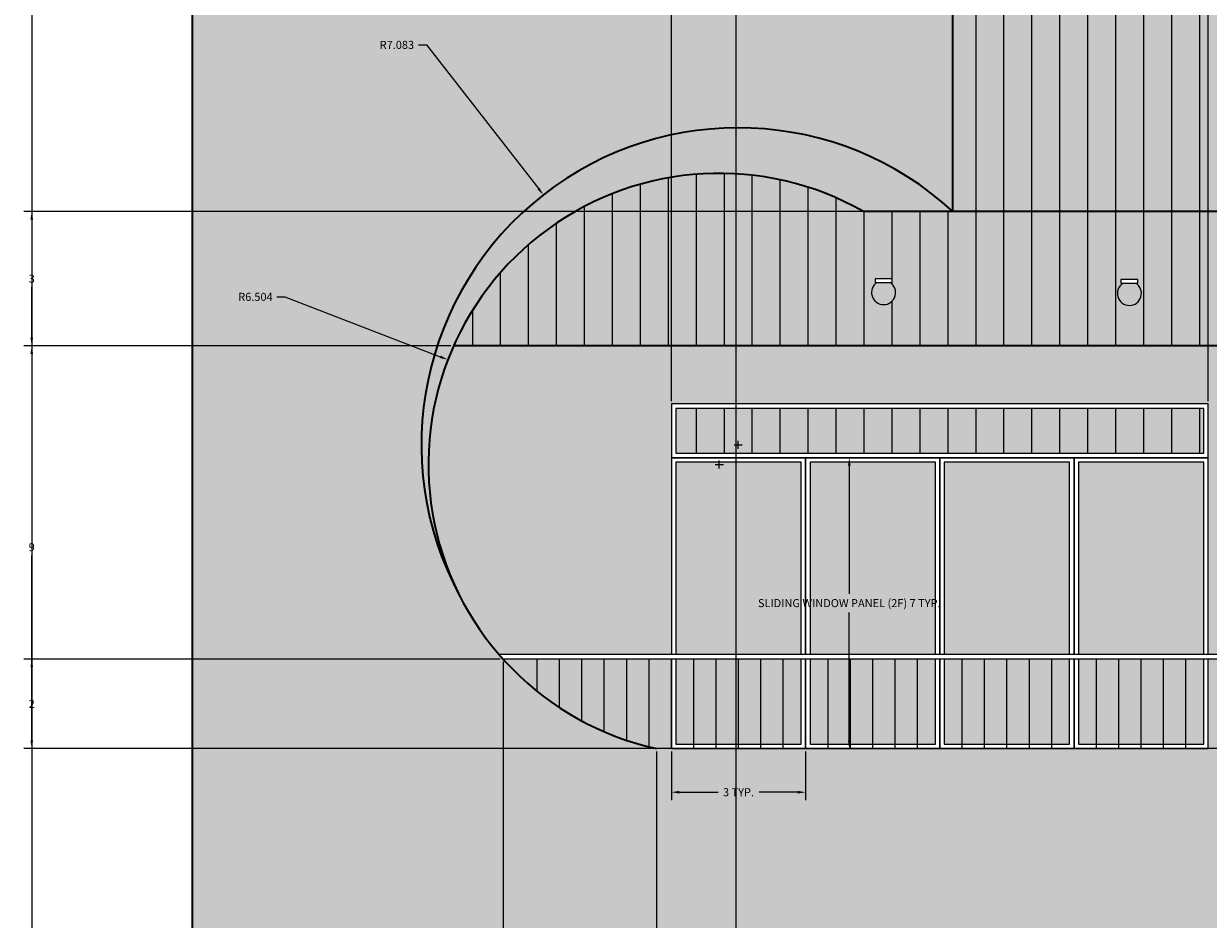
# Model space of a CAD drawing. Units: inches. Extents: x 18 to 59.8, y 2.7 to 81.2.
# Tile 7 of 9: x 18.1 to 44.6, y 45.6 to 65.6. Entities that reach past the tile are written whole.
import ezdxf

# ---------------------------------------------------------------- set-up
doc = ezdxf.new("R2010")
doc.units = ezdxf.units.IN
doc.header["$MEASUREMENT"] = 0
for name, color, linetype, lineweight in [('A-ANNO-DIMS', 2, 'Continuous', 18), ('A-ELEV', 7, 'Continuous', 35), ('A-ELEV-PATT', 8, 'Continuous', 13), ('A-ELEV-RAIL', 7, 'Continuous', 18), ('A-GLAZ', 4, 'Continuous', 25), ('E-LITE', 2, 'Continuous', 18)]:
    doc.layers.add(name, color=color, linetype=linetype, lineweight=lineweight)
doc.styles.get("Standard").update_dxf_attribs({"font": 'arial.ttf'})
doc.dimstyles.get("Standard").update_dxf_attribs({"dimtxt": 0.18, "dimasz": 0.18, "dimexe": 0.18, "dimexo": 0.0625, "dimgap": 0.09, "dimtad": 0, "dimtih": 1, "dimtoh": 1, "dimdec": 1, "dimzin": 0, "dimdsep": 46, "dimlunit": 3, "dimtxsty": 'Standard', "dimcen": 0.09, "dimadec": 0, "dimazin": 0, "dimtfac": 1, "dimtdec": 1, "dimtofl": 0, "dimtmove": 0, "dimatfit": 3, "dimfxl": 1, "dimtolj": 1, "dimtzin": 0, "dimarcsym": 0})

# ---------------------------------------------------------------- blocks, each defined once
blk = doc.blocks.new('LIGHT-CEILING-SPOT')
blk.add_lwpolyline([(0.079, 0.497), (0.459, 0.497), (0.459, 0.579), (0.079, 0.579)], close=True)
blk.add_arc((0.269, 0.269), 0.269, 122.0956, 57.9044)
blk = doc.blocks.new('WIN-SLIDING-PANEL-2F')
for points in [[(3, 2.1), (3, 6.5), (0, 6.5), (0, 2.1)], [(2.9, 2.1), (2.9, 6.4), (0.1, 6.4), (0.1, 2.1)], [(0, 2), (0, 0), (3, 0), (3, 2)], [(0.1, 2), (0.1, 0.1), (2.9, 0.1), (2.9, 2)]]:
    blk.add_lwpolyline(points)
blk = doc.blocks.new('*D6')
at = {"layer": 'A-ANNO-DIMS', "color": 0, "lineweight": -2, "transparency": 16777216}
for p, q in [((35.63, 55.941), (36.722, 55.941)), ((36.542, 55.761), (36.542, 52.899)), ((36.542, 49.621), (36.542, 52.483)), ((35.63, 49.441), (36.722, 49.441))]:
    blk.add_line(p, q, dxfattribs=at)
at = {"layer": 'A-ANNO-DIMS', "color": 0, "transparency": 16777216}
for points in [[(36.512, 55.761), (36.572, 55.761), (36.542, 55.941)], [(36.512, 49.621), (36.572, 49.621), (36.542, 49.441)]]:
    blk.add_solid(points, dxfattribs=at)
at = {"layer": 'Defpoints', "color": 0, "transparency": 16777216}
for p in [(35.567, 55.941), (36.542, 55.941), (35.567, 49.441)]:
    blk.add_point(p, dxfattribs=at)
at = {"layer": 'A-ANNO-DIMS', "color": 0, "transparency": 16777216, "insert": (36.542, 52.691), "char_height": 0.18, "attachment_point": 5}
blk.add_mtext('\\A1;SLIDING WINDOW PANEL (2F) 7 TYP.', dxfattribs=at)
blk = doc.blocks.new('*D7')
at = {"layer": 'A-ANNO-DIMS', "color": 0, "lineweight": -2, "transparency": 16777216}
for p, q in [((32.567, 49.378), (32.567, 48.286)), ((35.567, 49.378), (35.567, 48.286)), ((32.747, 48.466), (33.609, 48.466)), ((35.387, 48.466), (34.525, 48.466))]:
    blk.add_line(p, q, dxfattribs=at)
at = {"layer": 'A-ANNO-DIMS', "color": 0, "transparency": 16777216}
for points in [[(32.747, 48.496), (32.747, 48.436), (32.567, 48.466)], [(35.387, 48.496), (35.387, 48.436), (35.567, 48.466)]]:
    blk.add_solid(points, dxfattribs=at)
at = {"layer": 'Defpoints', "color": 0, "transparency": 16777216}
for p in [(32.567, 49.441), (35.567, 49.441), (35.567, 48.466)]:
    blk.add_point(p, dxfattribs=at)
at = {"layer": 'A-ANNO-DIMS', "color": 0, "transparency": 16777216, "insert": (34.067, 48.466), "char_height": 0.18, "attachment_point": 5}
blk.add_mtext('\\A1;3 TYP.', dxfattribs=at)
blk = doc.blocks.new('*D14')
at = {"layer": 'A-ANNO-DIMS', "color": 0, "lineweight": -2, "transparency": 16777216}
for p, q in [((21.797, 77.441), (18.09, 77.441)), ((18.27, 77.261), (18.27, 42.121)), ((18.27, 6.621), (18.27, 41.76)), ((21.797, 6.441), (18.09, 6.441))]:
    blk.add_line(p, q, dxfattribs=at)
at = {"layer": 'A-ANNO-DIMS', "color": 0, "transparency": 16777216}
for points in [[(18.24, 77.261), (18.3, 77.261), (18.27, 77.441)], [(18.24, 6.621), (18.3, 6.621), (18.27, 6.441)]]:
    blk.add_solid(points, dxfattribs=at)
at = {"layer": 'Defpoints', "color": 0, "transparency": 16777216}
for p in [(18.27, 77.441), (21.86, 77.441), (21.86, 6.441)]:
    blk.add_point(p, dxfattribs=at)
at = {"layer": 'A-ANNO-DIMS', "color": 0, "transparency": 16777216, "insert": (18.27, 41.941), "char_height": 0.18, "attachment_point": 5}
blk.add_mtext('\\A1;71', dxfattribs=at)
blk = doc.blocks.new('*D51')
at = {"layer": 'A-ANNO-DIMS', "color": 0, "lineweight": -2, "transparency": 16777216}
for p, q in [((34.012, 44.503), (34.012, 81.211)), ((34.192, 81.031), (40.98, 81.031)), ((48.68, 81.031), (41.891, 81.031)), ((48.86, 43.503), (48.86, 81.211))]:
    blk.add_line(p, q, dxfattribs=at)
at = {"layer": 'A-ANNO-DIMS', "color": 0, "transparency": 16777216}
for points in [[(34.192, 81.061), (34.192, 81.001), (34.012, 81.031)], [(48.68, 81.061), (48.68, 81.001), (48.86, 81.031)]]:
    blk.add_solid(points, dxfattribs=at)
at = {"layer": 'Defpoints', "color": 0, "transparency": 16777216}
for p in [(48.86, 81.031), (34.012, 44.441), (48.86, 43.441)]:
    blk.add_point(p, dxfattribs=at)
at = {"layer": 'A-ANNO-DIMS', "color": 0, "transparency": 16777216, "insert": (41.436, 81.031), "char_height": 0.18, "attachment_point": 5}
blk.add_mtext('\\A1;14.848', dxfattribs=at)
blk = doc.blocks.new('*D59')
at = {"layer": 'A-ANNO-DIMS', "color": 0, "lineweight": -2, "transparency": 16777216}
for p, q in [((27.636, 58.441), (18.09, 58.441)), ((18.27, 58.261), (18.27, 54.123)), ((18.27, 49.621), (18.27, 53.759)), ((32.171, 49.441), (18.09, 49.441))]:
    blk.add_line(p, q, dxfattribs=at)
at = {"layer": 'A-ANNO-DIMS', "color": 0, "transparency": 16777216}
for points in [[(18.24, 58.261), (18.3, 58.261), (18.27, 58.441)], [(18.24, 49.621), (18.3, 49.621), (18.27, 49.441)]]:
    blk.add_solid(points, dxfattribs=at)
at = {"layer": 'Defpoints', "color": 0, "transparency": 16777216}
for p in [(18.27, 58.441), (27.699, 58.441), (32.234, 49.441)]:
    blk.add_point(p, dxfattribs=at)
at = {"layer": 'A-ANNO-DIMS', "color": 0, "transparency": 16777216, "insert": (18.27, 53.941), "char_height": 0.18, "attachment_point": 5}
blk.add_mtext('\\A1;9', dxfattribs=at)
blk = doc.blocks.new('*D60')
at = {"layer": 'A-ANNO-DIMS', "color": 0, "lineweight": -2, "transparency": 16777216}
for p, q in [((38.797, 61.441), (18.09, 61.441)), ((18.27, 61.261), (18.27, 60.123)), ((18.27, 58.621), (18.27, 59.759)), ((27.636, 58.441), (18.09, 58.441))]:
    blk.add_line(p, q, dxfattribs=at)
at = {"layer": 'A-ANNO-DIMS', "color": 0, "transparency": 16777216}
for points in [[(18.24, 61.261), (18.3, 61.261), (18.27, 61.441)], [(18.24, 58.621), (18.3, 58.621), (18.27, 58.441)]]:
    blk.add_solid(points, dxfattribs=at)
at = {"layer": 'Defpoints', "color": 0, "transparency": 16777216}
for p in [(18.27, 61.441), (38.86, 61.441), (27.699, 58.441)]:
    blk.add_point(p, dxfattribs=at)
at = {"layer": 'A-ANNO-DIMS', "color": 0, "transparency": 16777216, "insert": (18.27, 59.941), "char_height": 0.18, "attachment_point": 5}
blk.add_mtext('\\A1;3', dxfattribs=at)
blk = doc.blocks.new('*D61')
at = {"layer": 'A-ANNO-DIMS', "color": 0, "lineweight": -2, "transparency": 16777216}
for p, q in [((32.234, 49.378), (32.234, 2.671)), ((47.86, 49.378), (47.86, 2.671)), ((32.414, 2.851), (39.592, 2.851)), ((47.68, 2.851), (40.502, 2.851))]:
    blk.add_line(p, q, dxfattribs=at)
at = {"layer": 'A-ANNO-DIMS', "color": 0, "transparency": 16777216}
for points in [[(32.414, 2.881), (32.414, 2.821), (32.234, 2.851)], [(47.68, 2.881), (47.68, 2.821), (47.86, 2.851)]]:
    blk.add_solid(points, dxfattribs=at)
at = {"layer": 'Defpoints', "color": 0, "transparency": 16777216}
for p in [(32.234, 49.441), (47.86, 49.441), (47.86, 2.851)]:
    blk.add_point(p, dxfattribs=at)
at = {"layer": 'A-ANNO-DIMS', "color": 0, "transparency": 16777216, "insert": (40.047, 2.851), "char_height": 0.18, "attachment_point": 5}
blk.add_mtext('\\A1;15.626', dxfattribs=at)
blk = doc.blocks.new('*D62')
at = {"layer": 'A-ANNO-DIMS', "color": 0, "lineweight": -2, "transparency": 16777216}
for p, q in [((32.567, 57.203), (32.567, 81.211)), ((32.747, 81.031), (38.358, 81.031)), ((44.387, 81.031), (38.777, 81.031)), ((44.567, 57.203), (44.567, 81.211))]:
    blk.add_line(p, q, dxfattribs=at)
at = {"layer": 'A-ANNO-DIMS', "color": 0, "transparency": 16777216}
for points in [[(32.747, 81.061), (32.747, 81.001), (32.567, 81.031)], [(44.387, 81.061), (44.387, 81.001), (44.567, 81.031)]]:
    blk.add_solid(points, dxfattribs=at)
at = {"layer": 'Defpoints', "color": 0, "transparency": 16777216}
for p in [(44.567, 81.031), (32.567, 57.141), (44.567, 57.141)]:
    blk.add_point(p, dxfattribs=at)
at = {"layer": 'A-ANNO-DIMS', "color": 0, "transparency": 16777216, "insert": (38.567, 81.031), "char_height": 0.18, "attachment_point": 5}
blk.add_mtext('\\A1;12', dxfattribs=at)
blk = doc.blocks.new('*D65')
at = {"layer": 'A-ANNO-DIMS', "color": 0, "lineweight": -2, "transparency": 16777216}
for p, q in [((28.741, 51.441), (18.09, 51.441)), ((18.27, 51.261), (18.27, 50.621)), ((18.27, 49.621), (18.27, 50.26)), ((32.171, 49.441), (18.09, 49.441))]:
    blk.add_line(p, q, dxfattribs=at)
at = {"layer": 'A-ANNO-DIMS', "color": 0, "transparency": 16777216}
for points in [[(18.24, 51.261), (18.3, 51.261), (18.27, 51.441)], [(18.24, 49.621), (18.3, 49.621), (18.27, 49.441)]]:
    blk.add_solid(points, dxfattribs=at)
at = {"layer": 'Defpoints', "color": 0, "transparency": 16777216}
for p in [(28.804, 51.441), (18.27, 49.441), (32.234, 49.441)]:
    blk.add_point(p, dxfattribs=at)
at = {"layer": 'A-ANNO-DIMS', "color": 0, "transparency": 16777216, "insert": (18.27, 50.441), "char_height": 0.18, "attachment_point": 5}
blk.add_mtext('\\A1;2', dxfattribs=at)
blk = doc.blocks.new('*D66')
at = {"layer": 'A-ANNO-DIMS', "color": 0, "lineweight": -2, "transparency": 16777216}
for p, q in [((28.804, 51.378), (28.804, 2.671)), ((48.567, 51.179), (48.567, 2.671)), ((28.984, 2.851), (38.231, 2.851)), ((48.387, 2.851), (39.14, 2.851))]:
    blk.add_line(p, q, dxfattribs=at)
at = {"layer": 'A-ANNO-DIMS', "color": 0, "transparency": 16777216}
for points in [[(28.984, 2.881), (28.984, 2.821), (28.804, 2.851)], [(48.387, 2.881), (48.387, 2.821), (48.567, 2.851)]]:
    blk.add_solid(points, dxfattribs=at)
at = {"layer": 'Defpoints', "color": 0, "transparency": 16777216}
for p in [(28.804, 51.441), (48.567, 51.242), (48.567, 2.851)]:
    blk.add_point(p, dxfattribs=at)
at = {"layer": 'A-ANNO-DIMS', "color": 0, "transparency": 16777216, "insert": (38.685, 2.851), "char_height": 0.18, "attachment_point": 5}
blk.add_mtext('\\A1;19.764', dxfattribs=at)
blk = doc.blocks.new('*D72')
at = {"layer": 'A-ANNO-DIMS', "color": 0, "lineweight": -2, "transparency": 16777216}
for p, q in [((26.911, 65.165), (27.091, 65.165)), ((27.091, 65.165), (29.594, 61.956)), ((33.972, 56.229), (34.152, 56.229)), ((34.062, 56.139), (34.062, 56.319))]:
    blk.add_line(p, q, dxfattribs=at)
at = {"layer": 'A-ANNO-DIMS', "color": 0, "transparency": 16777216}
blk.add_solid([(29.618, 61.974), (29.571, 61.937), (29.705, 61.814)], dxfattribs=at)
at = {"layer": 'Defpoints', "color": 0, "transparency": 16777216}
for p in [(29.705, 61.814), (34.062, 56.229)]:
    blk.add_point(p, dxfattribs=at)
at = {"layer": 'A-ANNO-DIMS', "color": 0, "transparency": 16777216, "insert": (26.431, 65.165), "char_height": 0.18, "attachment_point": 5}
blk.add_mtext('\\A1;R7.083', dxfattribs=at)
blk = doc.blocks.new('*D73')
at = {"layer": 'A-ANNO-DIMS', "color": 0, "lineweight": -2, "transparency": 16777216}
for p, q in [((23.749, 59.535), (23.929, 59.535)), ((23.929, 59.535), (27.402, 58.196)), ((33.638, 55.701), (33.638, 55.881)), ((33.548, 55.791), (33.728, 55.791))]:
    blk.add_line(p, q, dxfattribs=at)
at = {"layer": 'A-ANNO-DIMS', "color": 0, "transparency": 16777216}
blk.add_solid([(27.413, 58.224), (27.391, 58.168), (27.57, 58.131)], dxfattribs=at)
at = {"layer": 'Defpoints', "color": 0, "transparency": 16777216}
for p in [(27.57, 58.131), (33.638, 55.791)]:
    blk.add_point(p, dxfattribs=at)
at = {"layer": 'A-ANNO-DIMS', "color": 0, "transparency": 16777216, "insert": (23.27, 59.535), "char_height": 0.18, "attachment_point": 5}
blk.add_mtext('\\A1;R6.504', dxfattribs=at)

msp = doc.modelspace()

# ---------------------------------------------------------------- hatches: boundary and pattern name
at = {"layer": 'A-ELEV-PATT'}
h = msp.add_hatch(color=256, dxfattribs=at)
h.set_gradient(color1=(255, 255, 255), color2=(199, 200, 202))
h.paths.add_polyline_path([(38.86, 75.4521, 0.4125527), (36.86, 77.4407), (21.86, 77.4407), (21.86, 22.4407), (22.86, 22.4407), (48.86, 22.4407), (48.86, 30.9234, 0.4074473), (48.3302, 31.4407), (30.4061, 31.4407, -0.7603989), (34.0116, 44.4407), (47.86, 44.4407, -0.4142136), (48.86, 43.4407), (48.86, 48.4407, 0.4142136), (47.86, 49.4407), (32.2338, 49.4407, -0.2243142), (27.8411, 52.8427, -0.8480129), (38.86, 61.4407)])
h.paths.add_polyline_path([(55.86, 77.4407), (54.86, 77.4407), (54.86, 22.2407), (55.86, 22.2407)])
h.paths.add_polyline_path([(54.86, 51.5407), (53.4401, 51.5407), (53.4401, 29.6407), (54.86, 29.6407)])
h.paths.add_polyline_path([(54.86, 61.4407), (53.4401, 57.4407), (53.4401, 51.6407), (54.86, 51.6407)])
h.paths.add_polyline_path([(54.86, 29.4407), (54.471, 29.4407), (54.471, 22.2407), (54.86, 22.2407)])
h.paths.add_polyline_path([(55.5745, 22.2407), (54.86, 22.2407), (54.5745, 22.2407), (53.9347, 21.7925), (54.5877, 21.5495)])
h.paths.add_polyline_path([(54.5991, 21.5452), (53.9443, 21.789), (53.9443, 18.4407), (54.5991, 18.4407)])
h.paths.add_polyline_path([(53.9443, 21.789), (53.9347, 21.7925), (53.5816, 21.5452), (53.5816, 18.4407), (53.9443, 18.4407)])
h.paths.add_polyline_path([(53.3648, 20.6928), (52.8956, 21.0646), (52.8956, 18.4407), (53.3648, 18.4407)])
h.paths.add_polyline_path([(52.8956, 21.0646), (50.5775, 19.4407), (50.5775, 18.4407), (52.8956, 18.4407)])
h.paths.add_polyline_path([(53.5816, 21.5452), (52.8956, 21.0646), (53.3648, 20.6928), (53.5816, 20.8447)])
h.paths.add_polyline_path([(26.8109, 19.4407), (24.9672, 20.8407), (24.9672, 18.4407), (26.8109, 18.4407)])
h.paths.add_polyline_path([(24.9672, 20.8407), (24.4165, 20.8427), (24.4165, 18.4407), (24.9672, 18.4407)])
h.paths.add_polyline_path([(24.4165, 20.8427), (24.4165, 21.2589), (24.0588, 21.5305), (24.0301, 21.5183), (24.0301, 18.4407), (24.4165, 18.4407)])
h.paths.add_polyline_path([(24.0301, 21.5183), (23.4165, 21.2589), (23.4165, 18.4407), (24.0301, 18.4407)])
h.paths.add_polyline_path([(24.0301, 21.5183), (24.0588, 21.5305), (23.1234, 22.2407), (22.1234, 22.2407), (23.4165, 21.2589)])
h.paths.add_polyline_path([(24.4165, 21.2589), (24.4165, 20.8427), (24.9672, 20.8407)])
h.paths.add_polyline_path([(47.86, 18.4407), (29.86, 18.4407), (29.86, 6.4407), (30.86, 6.4407), (30.86, 17.4407), (38.86, 17.4407), (46.86, 17.4407), (46.86, 6.4407), (47.86, 6.4407)])
h.paths.add_polyline_path([(54.5756, 15.215), (54.5756, 6.4407), (55.86, 6.4407), (55.86, 18.4407), (47.86, 18.4407), (47.86, 6.4407), (49.1482, 6.4407), (49.1482, 15.215, -1)])
h = msp.add_hatch(color=256, dxfattribs=at)
h.paths.add_polyline_path([(27.8411, 52.8427, -0.7443789), (36.86, 61.4407), (38.86, 61.4407, 0.8480129)])
h.paths.add_polyline_path([(47.86, 44.4407), (34.0116, 44.4407, 0.7603989), (30.4061, 31.4407, -0.7376246), (34.0116, 43.4407), (47.86, 43.4407, -0.4142136), (48.86, 42.4407), (48.86, 43.4407, 0.4142136)])
h.paths.add_polyline_path([(54.5756, 15.215), (54.5756, 6.4407), (55.86, 6.4407), (55.86, 18.4407), (47.86, 18.4407), (47.86, 6.4407), (49.1482, 6.4407), (49.1482, 15.215, -1)])
h.paths.add_polyline_path([(47.86, 18.4407), (29.86, 18.4407), (29.86, 6.4407), (30.86, 6.4407), (30.86, 17.4407), (38.86, 17.4407), (46.86, 17.4407), (46.86, 6.4407), (47.86, 6.4407)])
h.paths.add_polyline_path([(55.86, 77.4407), (54.86, 77.4407), (54.86, 22.2407), (55.86, 22.2407)])
h = msp.add_hatch(color=256, dxfattribs=at)
h.dxf.hatch_style = 1
h.paths.add_polyline_path([(54.86, 69.4407), (38.86, 69.4407), (38.86, 61.4407), (54.86, 61.4407)])
h.paths.add_polyline_path([(54.86, 61.4407), (38.86, 61.4407), (36.86, 61.4407, 0.443414), (27.6986, 58.4407), (48.86, 58.4407), (48.86, 57.4407), (53.4401, 57.4407)])
h.paths.add_polyline_path([(37.4994, 59.9399), (37.4994, 59.8198, -2.4106499), (37.1187, 59.8198), (37.1187, 59.9399)], flags=16)
h.paths.add_polyline_path([(42.6125, 59.8012), (42.6125, 59.9213), (42.9933, 59.9213), (42.9933, 59.8012, -2.4106499)], flags=16)
h.paths.add_polyline_path([(49.5965, 59.971), (49.5965, 60.091), (49.9773, 60.091), (49.9773, 59.971, -2.4106499)], flags=16)
h.paths.add_polyline_path([(44.4671, 57.0407), (32.6671, 57.0407), (32.6671, 56.0407), (44.4671, 56.0407)])
h.paths.add_polyline_path([(47.86, 43.4407), (46.86, 43.4407), (34.0116, 43.4407, 0.2012983), (29.3481, 41.4407), (47.86, 41.4407, 1)])
h.paths.add_polyline_path([(36.5542, 42.5145), (36.5542, 42.6346), (36.9349, 42.6346), (36.9349, 42.5145, -2.4106499)], flags=16)
h.paths.add_polyline_path([(42.939, 42.5402), (42.939, 42.6603), (43.3198, 42.6603), (43.3198, 42.5402, -2.4106499)], flags=16)
h.paths.add_polyline_path([(54.471, 29.4407), (48.86, 29.4407), (48.86, 22.2407), (54.471, 22.2407)])
h.paths.add_polyline_path([(54.5745, 22.2407), (23.1234, 22.2407), (26.8109, 19.4407), (50.5775, 19.4407)])
h.paths.add_polyline_path([(54.5756, 15.215, 1), (49.1482, 15.215), (49.1482, 6.4407), (54.5756, 6.4407)])
h.paths.add_polyline_path([(49.8323, 12.602), (49.8323, 9.1225), (49.6657, 9.1225), (49.6657, 12.602)], flags=16)
h = msp.add_hatch(dxfattribs=at)
h.set_pattern_fill('ANSI31', color=256, scale=5, angle=45, style=0)
h.paths.add_polyline_path([(54.86, 69.4407), (38.86, 69.4407), (38.86, 61.4407), (54.86, 61.4407)])
h.paths.add_polyline_path([(54.86, 61.4407), (38.86, 61.4407), (36.86, 61.4407, 0.443414), (27.6986, 58.4407), (48.86, 58.4407), (48.86, 57.4407), (53.4401, 57.4407)])
h.paths.add_polyline_path([(37.1661, 59.8577), (37.1187, 59.8577), (37.1187, 59.9399), (37.4994, 59.9399), (37.4994, 59.8577), (37.452, 59.8577, -3.476462)], flags=16)
h.paths.add_polyline_path([(42.66, 59.8391), (42.6125, 59.8391), (42.6125, 59.9213), (42.9933, 59.9213), (42.9933, 59.8391), (42.9458, 59.8391, -3.476462)], flags=16)
h.paths.add_polyline_path([(49.644, 60.0088), (49.5965, 60.0088), (49.5965, 60.091), (49.9773, 60.091), (49.9773, 60.0088), (49.9298, 60.0088, -3.476462)], flags=16)
h.paths.add_polyline_path([(44.4671, 57.0407), (32.6671, 57.0407), (32.6671, 56.0407), (44.4671, 56.0407)])
h.paths.add_polyline_path([(47.86, 43.4407), (46.86, 43.4407), (34.0116, 43.4407, 0.2012983), (29.3481, 41.4407), (47.86, 41.4407, 1)])
h.paths.add_polyline_path([(36.6016, 42.5524), (36.5542, 42.5524), (36.5542, 42.6346), (36.9349, 42.6346), (36.9349, 42.5524), (36.8875, 42.5524, -3.476462)], flags=16)
h.paths.add_polyline_path([(42.9865, 42.578), (42.939, 42.578), (42.939, 42.6603), (43.3198, 42.6603), (43.3198, 42.578), (43.2723, 42.578, -3.476462)], flags=16)
h.paths.add_polyline_path([(54.471, 29.4407), (48.86, 29.4407), (48.86, 22.2407), (54.471, 22.2407)])
h.paths.add_polyline_path([(54.5745, 22.2407), (23.1234, 22.2407), (26.8109, 19.4407), (50.5775, 19.4407)])
h.paths.add_polyline_path([(54.5756, 15.215, 1), (49.1482, 15.215), (49.1482, 6.4407), (54.5756, 6.4407)])
h.paths.add_polyline_path([(49.8323, 9.1225), (49.6657, 9.1225), (49.6657, 12.602), (49.8323, 12.602)], flags=16)
h = msp.add_hatch(color=256, dxfattribs=at)
h.paths.add_polyline_path([(36.8875, 42.5524), (36.6016, 42.5524, 3.476462)])
h.paths.add_polyline_path([(43.2723, 42.578), (42.9865, 42.578, 3.476462)])
h.paths.add_polyline_path([(37.452, 59.8577), (37.1661, 59.8577, 3.476462)])
h.paths.add_polyline_path([(42.9458, 59.8391), (42.66, 59.8391, 3.476462)])
h.paths.add_polyline_path([(49.9298, 60.0088), (49.644, 60.0088, 3.476462)])
edge = h.paths.add_edge_path()
edge.add_ellipse((29.0313, 21.3107), major_axis=(-0.2068, 0), ratio=0.411448, start_angle=0, end_angle=360)
edge = h.paths.add_edge_path()
edge.add_ellipse((32.5919, 20.2963), major_axis=(-0.2068, 0), ratio=0.411448, start_angle=0, end_angle=360)
edge = h.paths.add_edge_path()
edge.add_ellipse((35.5044, 21.3908), major_axis=(-0.2068, 0), ratio=0.411448, start_angle=0, end_angle=360)
edge = h.paths.add_edge_path()
edge.add_ellipse((39.3877, 20.1968), major_axis=(-0.2068, 0), ratio=0.411448, start_angle=0, end_angle=360)
edge = h.paths.add_edge_path()
edge.add_ellipse((43.271, 21.3659), major_axis=(-0.2068, 0), ratio=0.411448, start_angle=0, end_angle=360)
edge = h.paths.add_edge_path()
edge.add_ellipse((47.3535, 20.1471), major_axis=(-0.2068, 0), ratio=0.411448, start_angle=0, end_angle=360)
at = {"layer": 'A-ELEV-PATT', "transparency": 33554620}
h = msp.add_hatch(color=256, dxfattribs=at)
h.set_gradient(color1=(147, 149, 152))
edge = h.paths.add_edge_path()
edge.add_line((32.5671, 55.9407), (32.5671, 57.1407))
edge.add_line((32.5671, 57.1407), (44.5671, 57.1407))
edge.add_line((44.5671, 57.1407), (44.5671, 55.9407))
edge.add_line((44.5671, 55.9407), (44.5671, 51.5407))
edge.add_line((44.5671, 51.5407), (47.9208, 51.5407))
edge.add_spline(control_points=[(47.9208, 51.5407), (48.1524, 51.5145), (48.3597, 51.3781), (48.5671, 51.2416)], knot_values=[0, 0, 0, 0, 0.7121901, 0.7121901, 0.7121901, 0.7121901], degree=3, periodic=0)
edge.add_line((48.5671, 51.2416), (48.5671, 49.1479))
edge.add_arc((47.86, 48.4407), 1, 5.73917, 45, ccw=False)
edge.add_line((48.855, 48.5407), (48.86, 48.5407))
edge.add_line((48.86, 48.5407), (48.86, 49.4407))
edge.add_line((48.86, 49.4407), (48.86, 58.4407))
edge.add_line((48.86, 58.4407), (27.6986, 58.4407))
edge.add_arc((33.6382, 55.7911), 6.5038, 155.95802, 220.80748)
edge.add_line((28.7154, 51.5407), (32.5671, 51.5407))
edge.add_line((32.5671, 51.5407), (32.5671, 55.9407))
edge = h.paths.add_edge_path()
edge.add_line((32.3302, 40.4407), (35.3302, 40.4407))
edge.add_line((35.3302, 40.4407), (38.3302, 40.4407))
edge.add_line((38.3302, 40.4407), (41.3302, 40.4407))
edge.add_line((41.3302, 40.4407), (44.3302, 40.4407))
edge.add_line((44.3302, 40.4407), (44.3302, 33.8336))
edge.add_line((44.3302, 33.8336), (47.6839, 33.8336))
edge.add_spline(control_points=[(47.6839, 33.8336), (47.9155, 33.8074), (48.1229, 33.671), (48.3302, 33.5345)], knot_values=[0, 0, 0, 0, 0.7121901, 0.7121901, 0.7121901, 0.7121901], degree=3, periodic=0)
edge.add_line((48.3302, 33.5345), (48.3302, 31.4407))
edge.add_arc((48.3304, 30.911), 0.5297, 1.3425, 90.01573, ccw=False)
edge.add_line((48.86, 30.9234), (48.86, 38.6846))
edge.add_line((48.86, 38.6846), (50.793, 38.6846))
edge.add_line((50.793, 38.6846), (50.793, 41.316))
edge.add_line((50.793, 41.316), (52.927, 41.316))
edge.add_line((52.927, 41.316), (52.927, 38.6846))
edge.add_line((52.927, 38.6846), (53.4401, 38.6846))
edge.add_line((53.4401, 38.6846), (53.4401, 48.4407))
edge.add_line((53.4401, 48.4407), (48.86, 48.4407))
edge.add_line((48.86, 48.4407), (48.86, 42.4407))
edge.add_arc((47.86, 42.4407), 1, -90, 0, ccw=False)
edge.add_line((47.86, 41.4407), (29.3481, 41.4407))
edge.add_arc((34.0631, 36.8836), 6.5573, 135.97541, 207.71831)
edge.add_line((28.2583, 33.8336), (32.3302, 33.8336))
edge.add_line((32.3302, 33.8336), (32.3302, 40.4407))
h.paths.add_polyline_path([(53.4401, 57.4407), (48.86, 57.4407), (48.86, 51.6407), (53.4401, 51.6407)])
h.paths.add_polyline_path([(29.5671, 51.4407), (28.8035, 51.4407, 0.040451), (29.5671, 50.7191)], flags=17)
h.paths.add_polyline_path([(30.0671, 51.4407), (29.5671, 51.4407), (29.5671, 50.7191, 0.0237787), (30.0671, 50.3554)], flags=17)
h.paths.add_polyline_path([(30.5671, 51.4407), (30.0671, 51.4407), (30.0671, 50.3554, 0.0223729), (30.5671, 50.0581)], flags=17)
h.paths.add_polyline_path([(31.0671, 51.4407), (30.5671, 51.4407), (30.5671, 50.0581, 0.021345), (31.0671, 49.8171)], flags=17)
h.paths.add_polyline_path([(31.5671, 51.4407), (31.0671, 51.4407), (31.0671, 49.8171, 0.0205858), (31.5671, 49.6259)], flags=17)
h.paths.add_polyline_path([(32.0671, 51.4407), (31.5671, 51.4407), (31.5671, 49.6259, 0.0200299), (32.0671, 49.4799)], flags=17)
h.paths.add_polyline_path([(32.5671, 51.4407), (32.0671, 51.4407), (32.0671, 49.4799, 0.0065845), (32.2338, 49.4407), (32.5671, 49.4407)], flags=17)
h.paths.add_polyline_path([(45.0671, 51.4407), (44.5671, 51.4407), (44.5671, 49.4407), (45.0671, 49.4407)], flags=17)
h.paths.add_polyline_path([(45.5671, 51.4407), (45.0671, 51.4407), (45.0671, 49.4407), (45.5671, 49.4407)], flags=17)
h.paths.add_polyline_path([(46.0671, 51.4407), (45.5671, 51.4407), (45.5671, 49.4407), (46.0671, 49.4407)], flags=17)
h.paths.add_polyline_path([(46.5671, 51.4407), (46.0671, 51.4407), (46.0671, 49.4407), (46.5671, 49.4407)], flags=17)
h.paths.add_polyline_path([(47.0671, 51.4407), (46.5671, 51.4407), (46.5671, 49.4407), (47.0671, 49.4407)], flags=17)
h.paths.add_polyline_path([(47.5671, 51.4407), (47.0671, 51.4407), (47.0671, 49.4407), (47.5671, 49.4407)], flags=17)
edge = h.paths.add_edge_path(flags=17)
edge.add_spline(control_points=[(48.0671, 51.4184), (48.0217, 51.4311), (47.9752, 51.4389), (47.9273, 51.4407)], knot_values=[0.570104, 0.570104, 0.570104, 0.570104, 0.7151116, 0.7151116, 0.7151116, 0.7151116], degree=3, periodic=0)
edge.add_line((47.9273, 51.4407), (47.5671, 51.4407))
edge.add_line((47.5671, 51.4407), (47.5671, 49.4407))
edge.add_line((47.5671, 49.4407), (47.86, 49.4407))
edge.add_arc((47.86, 48.4407), 1, 78.04714, 90, ccw=False)
edge.add_line((48.0671, 49.4191), (48.0671, 51.4184))
edge = h.paths.add_edge_path(flags=17)
edge.add_spline(control_points=[(48.5671, 51.1212), (48.4062, 51.2449), (48.2454, 51.3687), (48.0671, 51.4184)], knot_values=[0, 0, 0, 0, 0.570104, 0.570104, 0.570104, 0.570104], degree=3, periodic=0)
edge.add_line((48.0671, 51.4184), (48.0671, 49.4191))
edge.add_arc((47.86, 48.4407), 1, 45, 78.04714, ccw=False)
edge.add_line((48.5671, 49.1479), (48.5671, 51.1212))
h.paths.add_polyline_path([(49.36, 51.5407), (48.86, 51.5407), (48.86, 49.4407), (48.86, 48.5407), (49.36, 48.5407)])
h.paths.add_polyline_path([(49.86, 51.5407), (49.36, 51.5407), (49.36, 48.5407), (49.86, 48.5407)])
h.paths.add_polyline_path([(50.36, 51.5407), (49.86, 51.5407), (49.86, 48.5407), (50.36, 48.5407)])
h.paths.add_polyline_path([(50.86, 51.5407), (50.36, 51.5407), (50.36, 48.5407), (50.86, 48.5407)])
h.paths.add_polyline_path([(51.36, 51.5407), (50.86, 51.5407), (50.86, 48.5407), (51.36, 48.5407)])
h.paths.add_polyline_path([(51.86, 51.5407), (51.36, 51.5407), (51.36, 48.5407), (51.86, 48.5407)])
h.paths.add_polyline_path([(52.36, 51.5407), (51.86, 51.5407), (51.86, 48.5407), (52.36, 48.5407)])
h.paths.add_polyline_path([(52.86, 51.5407), (52.36, 51.5407), (52.36, 48.5407), (52.86, 48.5407)])
h.paths.add_polyline_path([(53.36, 51.5407), (52.86, 51.5407), (52.86, 48.5407), (53.36, 48.5407)])
h.paths.add_polyline_path([(53.4401, 38.6846), (48.86, 38.6846), (48.86, 30.9234), (48.86, 29.6407), (53.4401, 29.6407)])
h.paths.add_polyline_path([(28.8302, 33.7336), (28.3119, 33.7336, 0.0364452), (28.8302, 32.9319)], flags=17)
h.paths.add_polyline_path([(29.3302, 33.7336), (28.8302, 33.7336), (28.8302, 32.9319, 0.0294201), (29.3302, 32.3451)], flags=17)
h.paths.add_polyline_path([(29.8302, 33.7336), (29.3302, 33.7336), (29.3302, 32.3451, 0.0261691), (29.8302, 31.8755)], flags=17)
h.paths.add_polyline_path([(30.3302, 33.7336), (29.8302, 33.7336), (29.8302, 31.8755, 0.0240263), (30.3302, 31.4925)], flags=17)
h.paths.add_polyline_path([(30.8302, 33.7336), (30.3302, 33.7336), (30.3302, 31.4925, 0.0035006), (30.4061, 31.4407), (30.8302, 31.4407)], flags=17)
h.paths.add_polyline_path([(31.3302, 33.7336), (30.8302, 33.7336), (30.8302, 31.4407), (31.3302, 31.4407)], flags=17)
h.paths.add_polyline_path([(31.8302, 33.7336), (31.3302, 33.7336), (31.3302, 31.4407), (31.8302, 31.4407)], flags=17)
h.paths.add_polyline_path([(32.3302, 33.7336), (31.8302, 33.7336), (31.8302, 31.4407), (32.3302, 31.4407)], flags=17)
h.paths.add_polyline_path([(44.8302, 33.7336), (44.3302, 33.7336), (44.3302, 31.4407), (44.8302, 31.4407)], flags=17)
h.paths.add_polyline_path([(45.3302, 33.7336), (44.8302, 33.7336), (44.8302, 31.4407), (45.3302, 31.4407)], flags=17)
h.paths.add_polyline_path([(45.8302, 33.7336), (45.3302, 33.7336), (45.3302, 31.4407), (45.8302, 31.4407)], flags=17)
h.paths.add_polyline_path([(46.3302, 33.7336), (45.8302, 33.7336), (45.8302, 31.4407), (46.3302, 31.4407)], flags=17)
h.paths.add_polyline_path([(46.8302, 33.7336), (46.3302, 33.7336), (46.3302, 31.4407), (46.8302, 31.4407)], flags=17)
h.paths.add_polyline_path([(47.3302, 33.7336), (46.8302, 33.7336), (46.8302, 31.4407), (47.3302, 31.4407)], flags=17)
edge = h.paths.add_edge_path(flags=16)
edge.add_spline(control_points=[(47.8302, 33.7113), (47.7849, 33.7239), (47.7384, 33.7318), (47.6905, 33.7336)], knot_values=[0.570104, 0.570104, 0.570104, 0.570104, 0.7151116, 0.7151116, 0.7151116, 0.7151116], degree=3, periodic=0)
edge.add_line((47.6905, 33.7336), (47.3302, 33.7336))
edge.add_line((47.3302, 33.7336), (47.3302, 31.4407))
edge.add_line((47.3302, 31.4407), (47.8302, 31.4407))
edge.add_line((47.8302, 31.4407), (47.8302, 33.7113))
h.paths.add_polyline_path([(48.86, 38.6846), (50.793, 38.6846), (50.793, 41.316), (52.927, 41.316), (52.927, 38.6846), (53.4401, 38.6846), (53.4401, 48.4407), (48.86, 48.4407), (48.86, 42.4407, -0.4142136), (47.86, 41.4407), (29.3481, 41.4407, 0.3236799), (28.2583, 33.8336), (32.3302, 33.8336), (32.3302, 40.4407), (35.3302, 40.4407), (38.3302, 40.4407), (41.3302, 40.4407), (44.3302, 40.4407), (44.3302, 33.8336), (28.2583, 33.8336, 0.0043267), (28.3119, 33.7336), (28.8302, 33.7336), (29.3302, 33.7336), (29.8302, 33.7336), (30.3302, 33.7336), (30.8302, 33.7336), (31.3302, 33.7336), (31.8302, 33.7336), (32.3302, 33.7336), (47.3302, 33.7336), (47.3302, 31.4407), (47.8302, 31.4407), (48.3302, 31.4407, -0.4074473), (48.86, 30.9234)])
edge = h.paths.add_edge_path(flags=0)
edge.add_spline(control_points=[(47.8302, 33.7113), (47.7849, 33.7239), (47.7384, 33.7318), (47.6905, 33.7336)], knot_values=[0.570104, 0.570104, 0.570104, 0.570104, 0.7151116, 0.7151116, 0.7151116, 0.7151116], degree=3, periodic=0)
edge.add_line((47.6905, 33.7336), (47.3302, 33.7336))
edge.add_line((47.3302, 33.7336), (47.3302, 31.4407))
edge.add_line((47.3302, 31.4407), (47.8302, 31.4407))
edge.add_line((47.8302, 31.4407), (47.8302, 33.7113))
at = {"layer": 'A-ELEV-PATT', "transparency": 33554618}
h = msp.add_hatch(color=256, dxfattribs=at)
h.set_gradient(color1=(173, 221, 247), rotation=20)
h.paths.add_polyline_path([(35.4671, 55.8407), (32.6671, 55.8407), (32.6671, 51.5407), (35.4671, 51.5407)])
h.paths.add_polyline_path([(38.4671, 55.8407), (35.6671, 55.8407), (35.6671, 51.5407), (38.4671, 51.5407)])
h.paths.add_polyline_path([(41.4671, 55.8407), (38.6671, 55.8407), (38.6671, 51.5407), (41.4671, 51.5407)])
h.paths.add_polyline_path([(44.4671, 55.8407), (41.6671, 55.8407), (41.6671, 51.5407), (44.4671, 51.5407)])
h.paths.add_polyline_path([(33.0671, 51.4407), (32.6671, 51.4407), (32.6671, 49.5407), (33.0671, 49.5407)])
h.paths.add_polyline_path([(33.5671, 51.4407), (33.0671, 51.4407), (33.0671, 49.5407), (33.5671, 49.5407)])
h.paths.add_polyline_path([(34.0671, 51.4407), (33.5671, 51.4407), (33.5671, 49.5407), (34.0671, 49.5407)])
h.paths.add_polyline_path([(34.5671, 51.4407), (34.0671, 51.4407), (34.0671, 49.5407), (34.5671, 49.5407)])
h.paths.add_polyline_path([(35.0671, 51.4407), (34.5671, 51.4407), (34.5671, 49.5407), (35.0671, 49.5407)])
h.paths.add_polyline_path([(35.4671, 51.4407), (35.0671, 51.4407), (35.0671, 49.5407), (35.4671, 49.5407)])
h.paths.add_polyline_path([(36.0671, 51.4407), (35.6671, 51.4407), (35.6671, 49.5407), (36.0671, 49.5407)])
h.paths.add_polyline_path([(36.5671, 51.4407), (36.0671, 51.4407), (36.0671, 49.5407), (36.5671, 49.5407)])
h.paths.add_polyline_path([(37.0671, 51.4407), (36.5671, 51.4407), (36.5671, 49.5407), (37.0671, 49.5407)])
h.paths.add_polyline_path([(37.5671, 51.4407), (37.0671, 51.4407), (37.0671, 49.5407), (37.5671, 49.5407)])
h.paths.add_polyline_path([(38.0671, 51.4407), (37.5671, 51.4407), (37.5671, 49.5407), (38.0671, 49.5407)])
h.paths.add_polyline_path([(38.4671, 51.4407), (38.0671, 51.4407), (38.0671, 49.5407), (38.4671, 49.5407)])
h.paths.add_polyline_path([(39.0671, 51.4407), (38.6671, 51.4407), (38.6671, 49.5407), (39.0671, 49.5407)])
h.paths.add_polyline_path([(39.5671, 51.4407), (39.0671, 51.4407), (39.0671, 49.5407), (39.5671, 49.5407)])
h.paths.add_polyline_path([(40.0671, 51.4407), (39.5671, 51.4407), (39.5671, 49.5407), (40.0671, 49.5407)])
h.paths.add_polyline_path([(40.5671, 51.4407), (40.0671, 51.4407), (40.0671, 49.5407), (40.5671, 49.5407)])
h.paths.add_polyline_path([(41.0671, 51.4407), (40.5671, 51.4407), (40.5671, 49.5407), (41.0671, 49.5407)])
h.paths.add_polyline_path([(41.4671, 51.4407), (41.0671, 51.4407), (41.0671, 49.5407), (41.4671, 49.5407)])
h.paths.add_polyline_path([(42.0671, 51.4407), (41.6671, 51.4407), (41.6671, 49.5407), (42.0671, 49.5407)])
h.paths.add_polyline_path([(42.5671, 51.4407), (42.0671, 51.4407), (42.0671, 49.5407), (42.5671, 49.5407)])
h.paths.add_polyline_path([(43.0671, 51.4407), (42.5671, 51.4407), (42.5671, 49.5407), (43.0671, 49.5407)])
h.paths.add_polyline_path([(43.5671, 51.4407), (43.0671, 51.4407), (43.0671, 49.5407), (43.5671, 49.5407)])
h.paths.add_polyline_path([(44.0671, 51.4407), (43.5671, 51.4407), (43.5671, 49.5407), (44.0671, 49.5407)])
h.paths.add_polyline_path([(44.4671, 51.4407), (44.0671, 51.4407), (44.0671, 49.5407), (44.4671, 49.5407)])

# ---------------------------------------------------------------- linework, layer by layer
at = {"layer": 'A-ELEV'}
for p, q in [((21.86, 22.2407), (21.86, 77.4407)), ((38.86, 61.4407), (38.86, 75.4521)), ((38.86, 61.4407), (36.86, 61.4407)), ((54.86, 61.4407), (38.86, 61.4407)), ((48.86, 58.4407), (27.6986, 58.4407))]:
    msp.add_line(p, q, dxfattribs=at)
for centre, radius, start, end in [((34.0625, 56.2293), 7.0834, 47.3684, 208.5619), ((33.6382, 55.7911), 6.5038, 60.30534, 257.53013)]:
    msp.add_arc(centre, radius, start, end, dxfattribs=at)
at = {"layer": 'A-ELEV-RAIL'}
for p, q in [((47.9208, 51.5407), (28.7154, 51.5407)), ((47.9273, 51.4407), (28.8035, 51.4407)), ((29.5671, 50.7191), (29.5671, 51.4407)), ((30.0671, 50.3554), (30.0671, 51.4407)), ((30.5671, 50.0581), (30.5671, 51.4407)), ((31.0671, 49.8171), (31.0671, 51.4407)), ((31.5671, 49.6259), (31.5671, 51.4407)), ((32.0671, 49.4799), (32.0671, 51.4407)), ((32.5671, 49.4407), (32.5671, 51.4407)), ((33.0671, 49.4407), (33.0671, 51.4407)), ((33.5671, 49.4407), (33.5671, 51.4407)), ((34.0671, 49.4407), (34.0671, 51.4407)), ((34.5671, 49.4407), (34.5671, 51.4407)), ((35.0671, 49.4407), (35.0671, 51.4407)), ((35.5671, 49.4407), (35.5671, 51.4407)), ((36.0671, 49.4407), (36.0671, 51.4407)), ((36.5671, 49.4407), (36.5671, 51.4407)), ((37.0671, 49.4407), (37.0671, 51.4407)), ((37.5671, 49.4407), (37.5671, 51.4407)), ((38.0671, 49.4407), (38.0671, 51.4407)), ((38.5671, 49.4407), (38.5671, 51.4407)), ((39.0671, 49.4407), (39.0671, 51.4407)), ((39.5671, 49.4407), (39.5671, 51.4407)), ((40.0671, 49.4407), (40.0671, 51.4407)), ((40.5671, 49.4407), (40.5671, 51.4407)), ((41.0671, 49.4407), (41.0671, 51.4407)), ((41.5671, 49.4407), (41.5671, 51.4407)), ((42.0671, 49.4407), (42.0671, 51.4407)), ((42.5671, 49.4407), (42.5671, 51.4407)), ((43.0671, 49.4407), (43.0671, 51.4407)), ((43.5671, 49.4407), (43.5671, 51.4407)), ((44.0671, 49.4407), (44.0671, 51.4407)), ((44.5671, 49.4407), (44.5671, 51.4407)), ((47.86, 49.4407), (32.2338, 49.4407))]:
    msp.add_line(p, q, dxfattribs=at)
at = {"layer": 'A-GLAZ'}
for points in [[(32.5671, 55.9407), (44.5671, 55.9407), (44.5671, 57.1407), (32.5671, 57.1407)], [(32.6671, 56.0407), (44.4671, 56.0407), (44.4671, 57.0407), (32.6671, 57.0407)]]:
    msp.add_lwpolyline(points, close=True, dxfattribs=at)

# ---------------------------------------------------------------- block references
for p in [(32.567, 49.441), (35.567, 49.441), (38.567, 49.441), (41.567, 49.441)]:
    msp.add_blockref('WIN-SLIDING-PANEL-2F', p, dxfattribs=at)
at = {"layer": 'E-LITE'}
for p in [(37.04, 59.361), (42.5339, 59.3424)]:
    msp.add_blockref('LIGHT-CEILING-SPOT', p, dxfattribs=at)

# ---------------------------------------------------------------- dimensions: what is measured, and where the dimension line sits
at = {"layer": 'A-ANNO-DIMS'}
for base, p1, p2, override, picture, middle in [((44.5671, 81.0307), (32.5671, 57.1407), (44.5671, 57.1407), {"dimdec": 0, "dimlfac": 1, "dimrnd": 0, "dimzin": 0, "dimdsep": 46, "dimlunit": 2}, '*D62', (38.5671, 81.0307)), ((48.86, 81.0307), (34.0116, 44.4407), (48.86, 43.4407), {"dimdec": 3, "dimlfac": 1, "dimrnd": 0, "dimzin": 0, "dimdsep": 46, "dimlunit": 2}, '*D51', (41.4358, 81.0307)), ((48.5671, 2.8507), (28.8035, 51.4407), (48.5671, 51.2416), {"dimdec": 3, "dimlfac": 1, "dimrnd": 0, "dimzin": 0, "dimdsep": 46, "dimlunit": 2}, '*D66', (38.6853, 2.8507)), ((47.86, 2.8507), (32.2338, 49.4407), (47.86, 49.4407), {"dimdec": 3, "dimlfac": 1, "dimrnd": 0, "dimzin": 0, "dimdsep": 46, "dimlunit": 2}, '*D61', (40.0469, 2.8507))]:
    dim = msp.add_linear_dim(base=base, p1=p1, p2=p2, dimstyle='Standard', override=override, dxfattribs=at)
    dim.commit()
    dim.dimension.update_dxf_attribs({"geometry": picture, "text_midpoint": middle})
for base, p1, p2, picture, middle in [((18.27, 77.4407), (21.86, 6.4407), (21.86, 77.4407), '*D14', (18.27, 41.9407)), ((18.27, 61.4407), (27.6986, 58.4407), (38.86, 61.4407), '*D60', (18.27, 59.9407)), ((18.27, 58.4407), (32.2338, 49.4407), (27.6986, 58.4407), '*D59', (18.27, 53.9407)), ((18.27, 49.4407), (28.8035, 51.4407), (32.2338, 49.4407), '*D65', (18.27, 50.4407))]:
    dim = msp.add_linear_dim(base=base, p1=p1, p2=p2, angle=90, dimstyle='Standard', override={"dimdec": 0, "dimlfac": 1, "dimrnd": 0, "dimzin": 0, "dimdsep": 46, "dimlunit": 2}, dxfattribs=at)
    dim.commit()
    dim.dimension.update_dxf_attribs({"geometry": picture, "text_midpoint": middle})
for center, mpoint, picture, middle in [((34.0625, 56.2293), (29.7051, 61.8139), '*D72', (26.4308, 65.1647)), ((33.6382, 55.7911), (27.5699, 58.131), '*D73', (23.2695, 59.535))]:
    dim = msp.add_radius_dim(center=center, mpoint=mpoint, dimstyle='Standard', override={"dimdec": 3, "dimlfac": 1, "dimrnd": 0, "dimzin": 0, "dimdsep": 46, "dimlunit": 2}, dxfattribs=at)
    dim.commit()
    dim.dimension.update_dxf_attribs({"geometry": picture, "text_midpoint": middle, "dimtype": 164})
dim = msp.add_linear_dim(base=(36.542077653, 55.9407475058), p1=(35.567077653, 49.4407475058), p2=(35.567077653, 55.9407475058), angle=90, text='SLIDING WINDOW PANEL (2F) <> TYP.', dimstyle='Standard', override={"dimdec": 0, "dimlfac": 1, "dimrnd": 0, "dimzin": 0, "dimdsep": 46, "dimlunit": 2}, dxfattribs=at)
dim.commit()
dim.dimension.update_dxf_attribs({"geometry": '*D6', "text_midpoint": (36.542077653, 52.6907475058)})
dim = msp.add_linear_dim(base=(35.5671, 48.4657), p1=(32.5671, 49.4407), p2=(35.5671, 49.4407), text='<> TYP.', dimstyle='Standard', override={"dimdec": 0, "dimlfac": 1, "dimrnd": 0, "dimzin": 0, "dimdsep": 46, "dimlunit": 2}, dxfattribs=at)
dim.commit()
dim.dimension.update_dxf_attribs({"geometry": '*D7', "text_midpoint": (34.0671, 48.4657)})

doc.saveas('drawing.dxf')
